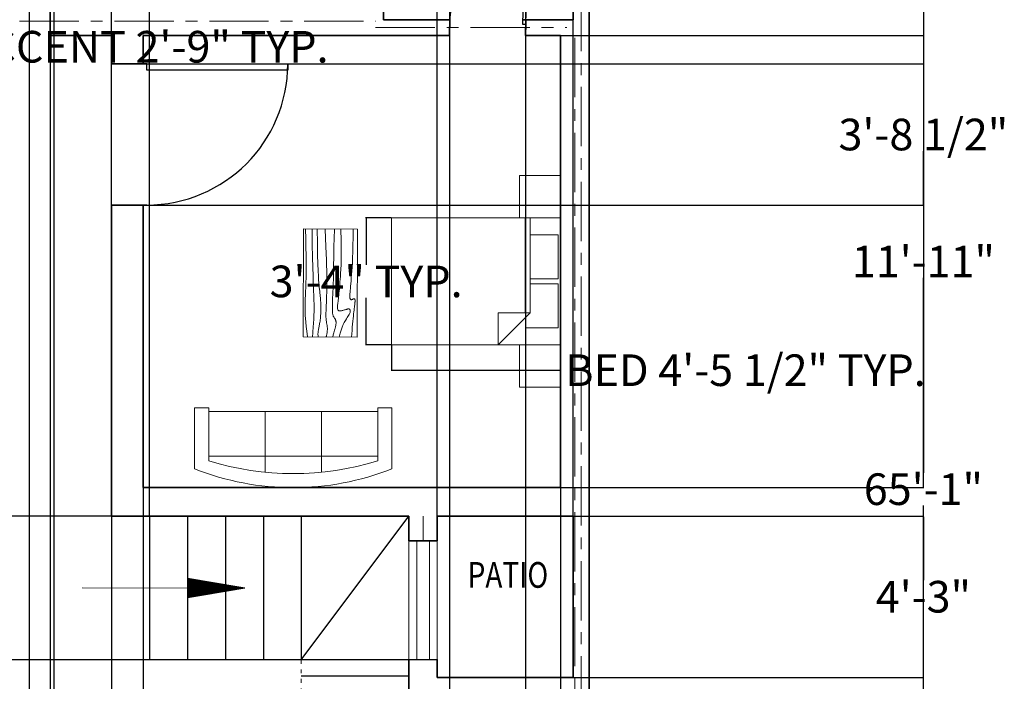
# Model space of a CAD drawing. Units: inches. Extents: x 541 to 1172, y -20 to 887.
# Tile 5 of 8: x 857 to 1169, y 378 to 588. Entities that reach past the tile are written whole.
import ezdxf

# ---------------------------------------------------------------- set-up
doc = ezdxf.new("R2010")
doc.units = ezdxf.units.IN
doc.header["$MEASUREMENT"] = 0
doc.linetypes.add('ACAD_ISO03W100', pattern=[30, 12, -18])
doc.linetypes.add('CENTER', pattern=[50.8, 31.75, -6.35, 6.35, -6.35])
doc.layers.get('0').update_dxf_attribs({"color": 70})
for name, color, linetype, lineweight in [('A-ANNO-DIMS', 2, 'Continuous', 18), ('A-ANNO-SYMB', 7, 'Continuous', 18), ('A-AREA-IDEN', 7, 'Continuous', 20), ('A-DOOR', 4, 'Continuous', 25), ('A-FLOR-STRS-HIDN', 131, 'ACAD_ISO03W100', 18), ('A-FURN', 30, 'Continuous', 18), ('A-WALL-CNTR', 1, 'CENTER', 13), ('STAIRS', 131, 'Continuous', 25), ('WALL', 7, 'Continuous', 35), ('WINDOW', 2, 'Continuous', 18)]:
    doc.layers.add(name, color=color, linetype=linetype, lineweight=lineweight)
doc.styles.get("Standard").update_dxf_attribs({"font": 'arial.ttf'})
doc.styles.add('YQ_DIM', font='SUPEROS.SHX', dxfattribs={"width": 0.8, "bigfont": 'HZDX.SHX'})
doc.dimstyles.get("Standard").update_dxf_attribs({"dimtxt": 10, "dimasz": 0.18, "dimexe": 0.18, "dimexo": 0.0625, "dimgap": 0.09, "dimtad": 0, "dimtih": 1, "dimtoh": 1, "dimdec": 1, "dimzin": 0, "dimdsep": 46, "dimlunit": 4, "dimtxsty": 'Standard', "dimcen": 0.09, "dimadec": 0, "dimazin": 0, "dimtfac": 1, "dimtdec": 1, "dimtofl": 0, "dimtmove": 0, "dimatfit": 3, "dimfxl": 1, "dimtolj": 1, "dimtzin": 0, "dimarcsym": 0})

# ---------------------------------------------------------------- blocks, each defined once
blk = doc.blocks.new('Bed - Queen')
for p, q in [((0, -80.00003), (0, 0)), ((0, 0), (59.99999, 0)), ((59.99999, 0), (59.99999, -80.00003)), ((7.99999, -1.2), (28.79998, -1.2)), ((7.99999, -14.4), (7.99999, -1.2)), ((28.79998, -1.2), (28.79998, -14.4)), ((31.19999, -1.2), (51.99999, -1.2)), ((31.19999, -14.4), (31.19999, -1.2)), ((51.99999, -1.2), (51.99999, -16.4)), ((0, -14.4), (44.8, -14.4)), ((44.8, -16.8), (0, -16.8)), ((59.99999, -29.6), (44.8, -14.4)), ((44.8, -14.4), (44.8, -29.6)), ((51.99999, -16.4), (46.79936, -16.4)), ((44.8, -29.6), (59.99999, -29.6)), ((59.99999, -80.00003), (0, -80.00003))]:
    blk.add_line(p, q)
blk = doc.blocks.new('Table - Rectangular Woodgrain 60 x 30 in.')
for p, q in [((0, 0), (0, -30)), ((60, 0), (0, 0)), ((60, -30), (60, 0)), ((0, -30), (60, -30))]:
    blk.add_line(p, q)
for points in [[(0, -2.4), (4.8155, -2.418), (9.0302, -2.4688), (12.709, -2.5477), (15.9167, -2.65), (18.7181, -2.7711), (21.1781, -2.9063), (23.3616, -3.0508), (25.3333, -3.2), (27.1477, -3.3495), (28.8172, -3.4958), (30.3437, -3.636), (31.7291, -3.7667), (32.9756, -3.8849), (34.0849, -3.9875), (35.059, -4.0714), (35.9, -4.1334), (36.6114, -4.1711), (37.2041, -4.1854), (37.6906, -4.1779), (38.0833, -4.15), (38.3948, -4.1034), (38.6375, -4.0396), (38.8239, -3.9602), (38.9666, -3.8667), (39.0764, -3.7608), (39.1573, -3.6448), (39.2116, -3.521), (39.2416, -3.3917), (39.2498, -3.2593), (39.2385, -3.1261), (39.21, -2.9944), (39.1666, -2.8667), (39.111, -2.7447), (39.0468, -2.6281), (38.978, -2.5163), (38.9083, -2.4083), (38.8418, -2.3035), (38.7823, -2.201), (38.7337, -2.1001), (38.7, -2), (38.6844, -1.9003), (38.6875, -1.8021), (38.7094, -1.707), (38.75, -1.6167), (38.8094, -1.5326), (38.8875, -1.4563), (38.9844, -1.3893), (39.1, -1.3333), (39.2351, -1.2896), (39.3937, -1.2583), (39.5804, -1.2396), (39.8, -1.2333), (40.057, -1.2396), (40.3562, -1.2583), (40.7023, -1.2896), (41.1, -1.3333), (41.5547, -1.3895), (42.0755, -1.4573), (42.6721, -1.5361), (43.3542, -1.625), (44.1316, -1.7233), (45.014, -1.8302), (46.0114, -1.9449), (47.1333, -2.0667), (48.3862, -2.1947), (49.7625, -2.3281), (51.2513, -2.4663), (52.8416, -2.6083), (54.5226, -2.7535), (56.2833, -2.9011), (58.1127, -3.0501), (60, -3.2)], [(0, -9.2), (6.5759, -9.0858), (11.9385, -9.0365), (16.2527, -9.0418), (19.6833, -9.0917), (22.3952, -9.1759), (24.5531, -9.2844), (26.322, -9.4069), (27.8666, -9.5333), (29.3241, -9.6553), (30.7203, -9.7719), (32.0532, -9.8837), (33.3208, -9.9917), (34.5213, -10.0965), (35.6526, -10.199), (36.7128, -10.2999), (37.7, -10.4), (38.6129, -10.4996), (39.4531, -10.5969), (40.223, -10.6895), (40.925, -10.775), (41.5613, -10.8512), (42.1344, -10.9156), (42.6465, -10.966), (43.1, -11), (43.4976, -11.0158), (43.8437, -11.0136), (44.143, -10.9942), (44.4, -10.9583), (44.6195, -10.9069), (44.8062, -10.8406), (44.9648, -10.7603), (45.1, -10.6667), (45.2155, -10.5598), (45.3114, -10.4365), (45.3871, -10.2929), (45.4416, -10.125), (45.4743, -9.929), (45.4844, -9.7011), (45.4709, -9.4371), (45.4333, -9.1333), (45.3716, -8.7883), (45.2896, -8.4104), (45.1919, -8.0107), (45.0833, -7.6), (44.9685, -7.1893), (44.8521, -6.7896), (44.7388, -6.4117), (44.6333, -6.0667), (44.54, -5.7628), (44.4614, -5.4979), (44.4001, -5.2675), (44.3583, -5.0667), (44.3384, -4.8909), (44.3427, -4.7354), (44.3736, -4.5956), (44.4333, -4.4667), (44.5236, -4.3453), (44.6427, -4.2333), (44.7884, -4.1339), (44.9583, -4.05), (45.1501, -3.9849), (45.3614, -3.9417), (45.59, -3.9234), (45.8333, -3.9333), (46.0915, -3.9749), (46.3734, -4.0531), (46.6906, -4.1736), (47.0542, -4.3417), (47.4756, -4.5629), (47.9661, -4.8427), (48.5372, -5.1866), (49.2, -5.6), (49.9676, -6.0844), (50.8594, -6.625), (51.8965, -7.2031), (53.1, -7.8), (54.491, -8.3969), (56.0906, -8.975), (57.9199, -9.5156), (60, -10)], [(0, -12.8), (5.1847, -12.9322), (9.6213, -13.0323), (13.3963, -13.1059), (16.5958, -13.1583), (19.3063, -13.1952), (21.614, -13.2219), (23.6054, -13.2439), (25.3666, -13.2667), (26.9728, -13.2947), (28.4531, -13.3281), (29.8256, -13.3663), (31.1083, -13.4083), (32.3191, -13.4535), (33.476, -13.501), (34.597, -13.5501), (35.7, -13.6), (36.7984, -13.6497), (37.8875, -13.6979), (38.9578, -13.743), (40, -13.7833), (41.0047, -13.8174), (41.9625, -13.8438), (42.864, -13.8607), (43.7, -13.8667), (44.4631, -13.8604), (45.1552, -13.8417), (45.7801, -13.8104), (46.3416, -13.7667), (46.8439, -13.7104), (47.2906, -13.6417), (47.6858, -13.5604), (48.0333, -13.4667), (48.3375, -13.3608), (48.6042, -13.2448), (48.8396, -13.121), (49.05, -12.9917), (49.2417, -12.8593), (49.4208, -12.7261), (49.5937, -12.5944), (49.7667, -12.4667), (49.9452, -12.3451), (50.1323, -12.2313), (50.3303, -12.1268), (50.5416, -12.0333), (50.7686, -11.9524), (51.0135, -11.8854), (51.2788, -11.8341), (51.5666, -11.8), (51.8785, -11.7843), (52.2116, -11.7865), (52.562, -11.8059), (52.926, -11.8417), (53.2998, -11.8931), (53.6795, -11.9594), (54.0614, -12.0397), (54.4416, -12.1333), (54.8223, -12.2401), (55.2293, -12.3625), (55.6942, -12.5037), (56.2489, -12.6667), (56.9251, -12.8547), (57.7545, -13.0708), (58.7689, -13.3182), (60, -13.6)], [(0, -18), (5.124, -17.7273), (9.6609, -17.5057), (13.6705, -17.3303), (17.2125, -17.1958), (20.3467, -17.0973), (23.1328, -17.0297), (25.6307, -16.9878), (27.9, -16.9667), (29.9928, -16.9617), (31.9302, -16.9703), (33.7254, -16.9907), (35.3917, -17.0208), (36.9423, -17.0588), (38.3906, -17.1026), (39.7499, -17.1503), (41.0333, -17.2), (42.2519, -17.2496), (43.4073, -17.2969), (44.4986, -17.3395), (45.525, -17.375), (46.4858, -17.4012), (47.3802, -17.4156), (48.2074, -17.416), (48.9667, -17.4), (49.6583, -17.3662), (50.2872, -17.3167), (50.8595, -17.2547), (51.3812, -17.1833), (51.8584, -17.1057), (52.2971, -17.025), (52.7034, -16.9443), (53.0833, -16.8667), (53.443, -16.7951), (53.789, -16.7313), (54.128, -16.6768), (54.4666, -16.6334), (54.8115, -16.6024), (55.1693, -16.5854), (55.5465, -16.5841), (55.95, -16.6), (56.3828, -16.6337), (56.8346, -16.6823), (57.2915, -16.7418), (57.7396, -16.8084), (58.165, -16.878), (58.5539, -16.9469), (58.8924, -17.0111), (59.1666, -17.0667), (59.3679, -17.1107), (59.5078, -17.1438), (59.6032, -17.1675), (59.6708, -17.1833), (59.7275, -17.193), (59.7901, -17.1979), (59.8753, -17.1998), (60, -17.2)], [(0, -22.4), (8.0098, -22.2501), (14.4094, -22.1011), (19.4168, -21.9535), (23.25, -21.8083), (26.1269, -21.6663), (28.2656, -21.5281), (29.884, -21.3947), (31.2, -21.2667), (32.3967, -21.1448), (33.5172, -21.0292), (34.5697, -20.9198), (35.5625, -20.8167), (36.5037, -20.7198), (37.4015, -20.6292), (38.2642, -20.5448), (39.1, -20.4667), (39.9164, -20.3951), (40.7187, -20.3313), (41.5117, -20.2768), (42.3, -20.2333), (43.0883, -20.2024), (43.8812, -20.1854), (44.6836, -20.1841), (45.5, -20.2), (46.3328, -20.234), (47.1747, -20.2844), (48.0163, -20.3488), (48.8479, -20.425), (49.66, -20.5106), (50.4429, -20.6031), (51.1872, -20.7004), (51.8833, -20.8), (52.5246, -20.8999), (53.1166, -20.9995), (53.6681, -21.0983), (54.1875, -21.1958), (54.6834, -21.2919), (55.1646, -21.3859), (55.6394, -21.4777), (56.1167, -21.5667), (56.6028, -21.6515), (57.0961, -21.7266), (57.5929, -21.7852), (58.0896, -21.8208), (58.5823, -21.8268), (59.0674, -21.7964), (59.5412, -21.723), (60, -21.6)], [(0, -25.2), (8.6355, -25.0504), (15.7026, -24.9031), (21.4049, -24.7606), (25.9458, -24.625), (29.529, -24.4988), (32.3578, -24.3844), (34.6359, -24.284), (36.5667, -24.2), (38.3213, -24.1341), (39.9417, -24.0854), (41.437, -24.0523), (42.8167, -24.0333), (44.0901, -24.0268), (45.2667, -24.0313), (46.3557, -24.0451), (47.3667, -24.0667), (48.309, -24.0947), (49.1928, -24.1287), (50.0284, -24.168), (50.826, -24.2125), (51.5959, -24.2617), (52.3483, -24.3151), (53.0935, -24.3725), (53.8417, -24.4334), (54.6009, -24.497), (55.3699, -24.561), (56.1454, -24.6226), (56.9239, -24.6792), (57.7021, -24.7279), (58.4764, -24.7662), (59.2435, -24.7911), (60, -24.8)], [(0, -28.8), (5.6867, -28.6681), (10.45, -28.5698), (14.407, -28.5012), (17.675, -28.4584), (20.3711, -28.4374), (22.6125, -28.4344), (24.5164, -28.4455), (26.2, -28.4667), (27.762, -28.4947), (29.2276, -28.5281), (30.6033, -28.5663), (31.8958, -28.6084), (33.1118, -28.6535), (34.2578, -28.7011), (35.3405, -28.7501), (36.3666, -28.8), (37.3443, -28.8497), (38.288, -28.8974), (39.2137, -28.9412), (40.1375, -28.9792), (41.0753, -29.0093), (42.0432, -29.0297), (43.0572, -29.0384), (44.1333, -29.0333), (45.2936, -29.0114), (46.5843, -28.9641), (48.0579, -28.8816), (49.7666, -28.7542), (51.7629, -28.5721), (54.0989, -28.3255), (56.8272, -28.0048), (60, -27.6)]]:
    blk.add_lwpolyline(points)
blk = doc.blocks.new('Sofa - Roundback 7 ft.')
for p, q in [((-12.00002, -32.4421), (-12.00003, -6.5971)), ((11.99997, -32.4421), (11.99998, -6.5971)), ((-36.000027, -34), (-36.000027, -11.4696)), ((35.99998, -34), (35.99998, -11.4696)), ((-35.999844, -13.3819), (35.9998, -13.3819)), ((-36.000027, -32.4421), (35.99998, -32.4421))]:
    blk.add_line(p, q)
for points in [[(-36.000027, -34), (-42.000027, -34), (-42.000027, -8)], [(41.99998, -8), (41.99998, -34), (35.99998, -34)]]:
    blk.add_lwpolyline(points)
for centre, radius, start, end in [((0, -114.25), 114.25, 68.43141, 111.5686), ((-0.00001, -127.1968), 121.1968, 72.72033, 107.2797)]:
    blk.add_arc(centre, radius, start, end)
blk = doc.blocks.new('*U25')
for p, q in [((-40, 0), (-40, 6)), ((0, 0), (0, 6))]:
    blk.add_line(p, q)
blk.add_lwpolyline([(0, 0), (0, -40), (-1.75, -40), (-1.75, 0)], close=True)
blk.add_arc((0, 0), 40, 180, 270)
blk = doc.blocks.new('*U23')
for p, q in [((0, 0), (0, -6)), ((40, 0), (40, -6))]:
    blk.add_line(p, q)
blk.add_lwpolyline([(0, 0), (0, 40), (1.75, 40), (1.75, 0)], close=True)
blk.add_arc((0, 0), 40, 0, 90)
blk = doc.blocks.new('FURN-NIGHTSTAND')
for p, q in [((0, 13.4), (0, 0)), ((0, 0), (13, 0))]:
    blk.add_line(p, q)
blk = doc.blocks.new('*D55')
at = {"layer": 'A-ANNO-DIMS', "color": 0, "lineweight": -2, "transparency": 16777216}
for p, q in [((974.8, 484.76), (974.8, 476.62)), ((1028.28, 484.76), (1028.28, 476.62)), ((974.98, 476.8), (1028.1, 476.8)), ((1028.28, 476.8), (1028.46, 476.8))]:
    blk.add_line(p, q, dxfattribs=at)
for points in [[(974.98, 476.83), (974.98, 476.77), (974.8, 476.8)], [(1028.1, 476.83), (1028.1, 476.77), (1028.28, 476.8)]]:
    blk.add_solid(points, dxfattribs=at)
at = {"layer": 'Defpoints', "color": 0, "lineweight": -2, "transparency": 16777216}
for p in [(974.8, 484.83), (1028.28, 484.83), (1028.28, 476.8)]:
    blk.add_point(p, dxfattribs=at)
at = {"layer": 'A-ANNO-DIMS', "color": 0, "transparency": 16777216, "insert": (1086.76, 476.8), "char_height": 10, "attachment_point": 5}
blk.add_mtext('\\A1;BED 4\'-5 1/2" TYP.', dxfattribs=at)
blk = doc.blocks.new('*D56')
at = {"layer": 'A-ANNO-DIMS', "color": 0, "lineweight": -2, "transparency": 16777216}
for p, q in [((974.74, 524.94), (966.6, 524.94)), ((966.78, 524.76), (966.78, 510.08)), ((966.78, 485.01), (966.78, 499.68)), ((974.74, 484.83), (966.6, 484.83))]:
    blk.add_line(p, q, dxfattribs=at)
for points in [[(966.75, 524.76), (966.81, 524.76), (966.78, 524.94)], [(966.75, 485.01), (966.81, 485.01), (966.78, 484.83)]]:
    blk.add_solid(points, dxfattribs=at)
at = {"layer": 'Defpoints', "color": 0, "lineweight": -2, "transparency": 16777216}
for p in [(974.8, 524.94), (966.78, 484.83), (974.8, 484.83)]:
    blk.add_point(p, dxfattribs=at)
at = {"layer": 'A-ANNO-DIMS', "color": 0, "transparency": 16777216, "insert": (966.78, 504.88), "char_height": 10, "attachment_point": 5}
blk.add_mtext('\\A1;3\'-4" TYP.', dxfattribs=at)
blk = doc.blocks.new('*D61')
at = {"layer": 'A-ANNO-DIMS', "color": 0, "lineweight": -2, "transparency": 16777216}
for p, q in [((802.49, 574.25), (802.49, 579.28)), ((835.27, 574.25), (835.27, 579.28)), ((802.67, 579.1), (835.09, 579.1)), ((835.27, 579.1), (835.45, 579.1))]:
    blk.add_line(p, q, dxfattribs=at)
for points in [[(802.67, 579.13), (802.67, 579.07), (802.49, 579.1)], [(835.09, 579.13), (835.09, 579.07), (835.27, 579.1)]]:
    blk.add_solid(points, dxfattribs=at)
at = {"layer": 'Defpoints', "color": 0, "lineweight": -2, "transparency": 16777216}
for p in [(835.27, 579.1), (802.49, 574.19), (835.27, 574.19)]:
    blk.add_point(p, dxfattribs=at)
at = {"layer": 'A-ANNO-DIMS', "color": 0, "transparency": 16777216, "insert": (896.96, 579.1), "char_height": 10, "attachment_point": 5}
blk.add_mtext('\\A1;ACCENT 2\'-9" TYP.', dxfattribs=at)
blk = doc.blocks.new('*D70')
at = {"layer": 'A-ANNO-DIMS', "color": 0, "lineweight": -2, "transparency": 16777216}
for p, q in [((1036.7, 829.68), (1143.21, 829.68)), ((1143.03, 829.5), (1143.03, 444.36)), ((1143.03, 48.83), (1143.03, 433.97)), ((1037.35, 48.65), (1143.21, 48.65))]:
    blk.add_line(p, q, dxfattribs=at)
for points in [[(1143, 829.5), (1143.06, 829.5), (1143.03, 829.68)], [(1143, 48.83), (1143.06, 48.83), (1143.03, 48.65)]]:
    blk.add_solid(points, dxfattribs=at)
at = {"layer": 'Defpoints', "color": 0, "lineweight": -2, "transparency": 16777216}
for p in [(1036.64, 829.68), (1037.28, 48.65), (1143.03, 48.65)]:
    blk.add_point(p, dxfattribs=at)
at = {"layer": 'A-ANNO-DIMS', "color": 0, "transparency": 16777216, "insert": (1143.03, 439.17), "char_height": 10, "attachment_point": 5}
blk.add_mtext('\\A1;65\'-1"', dxfattribs=at)
blk = doc.blocks.new('*D86')
at = {"layer": 'A-ANNO-DIMS', "color": 0, "lineweight": -2, "transparency": 16777216}
for p, q in [((896.28, 439.59), (896.28, -5.37)), ((1028.28, 439.59), (1028.28, -5.37)), ((896.46, -5.19), (945.49, -5.19)), ((1028.1, -5.19), (979.08, -5.19))]:
    blk.add_line(p, q, dxfattribs=at)
for points in [[(896.46, -5.16), (896.46, -5.22), (896.28, -5.19)], [(1028.1, -5.16), (1028.1, -5.22), (1028.28, -5.19)]]:
    blk.add_solid(points, dxfattribs=at)
at = {"layer": 'Defpoints', "color": 0, "lineweight": -2, "transparency": 16777216}
for p in [(896.28, 439.65), (1028.28, 439.65), (1028.28, -5.19)]:
    blk.add_point(p, dxfattribs=at)
at = {"layer": 'A-ANNO-DIMS', "color": 0, "transparency": 16777216, "insert": (962.28, -5.19), "char_height": 10, "attachment_point": 5}
blk.add_mtext('\\A1;11\'-0"', dxfattribs=at)
blk = doc.blocks.new('*D87')
at = {"layer": 'A-ANNO-DIMS', "color": 0, "lineweight": -2, "transparency": 16777216}
for p, q in [((1028.35, 582.65), (1143.21, 582.65)), ((1143.03, 582.47), (1143.03, 516.26)), ((1143.03, 439.83), (1143.03, 506.04)), ((1028.35, 439.65), (1143.21, 439.65))]:
    blk.add_line(p, q, dxfattribs=at)
for points in [[(1143, 582.47), (1143.06, 582.47), (1143.03, 582.65)], [(1143, 439.83), (1143.06, 439.83), (1143.03, 439.65)]]:
    blk.add_solid(points, dxfattribs=at)
at = {"layer": 'Defpoints', "color": 0, "lineweight": -2, "transparency": 16777216}
for p in [(1028.28, 582.65), (1143.03, 582.65), (1028.28, 439.65)]:
    blk.add_point(p, dxfattribs=at)
at = {"layer": 'A-ANNO-DIMS', "color": 0, "transparency": 16777216, "insert": (1143.03, 511.15), "char_height": 10, "attachment_point": 5}
blk.add_mtext('\\A1;11\'-11"', dxfattribs=at)
blk = doc.blocks.new('*D88')
at = {"layer": 'A-ANNO-DIMS', "color": 0, "lineweight": -2, "transparency": 16777216}
for p, q in [((1032.35, 430.65), (1143.21, 430.65)), ((1143.03, 430.47), (1143.03, 410.35)), ((1143.03, 379.83), (1143.03, 399.96)), ((1032.35, 379.65), (1143.21, 379.65))]:
    blk.add_line(p, q, dxfattribs=at)
for points in [[(1143, 430.47), (1143.06, 430.47), (1143.03, 430.65)], [(1143, 379.83), (1143.06, 379.83), (1143.03, 379.65)]]:
    blk.add_solid(points, dxfattribs=at)
at = {"layer": 'Defpoints', "color": 0, "lineweight": -2, "transparency": 16777216}
for p in [(1032.28, 430.65), (1032.28, 379.65), (1143.03, 379.65)]:
    blk.add_point(p, dxfattribs=at)
at = {"layer": 'A-ANNO-DIMS', "color": 0, "transparency": 16777216, "insert": (1143.03, 405.15), "char_height": 10, "attachment_point": 5}
blk.add_mtext('\\A1;4\'-3"', dxfattribs=at)
blk = doc.blocks.new('*D89')
at = {"layer": 'A-ANNO-DIMS', "color": 0, "lineweight": -2, "transparency": 16777216}
for p, q in [((989.28, 430.72), (989.28, 872.66)), ((989.46, 872.48), (997.41, 872.48)), ((1032.1, 872.48), (1024.16, 872.48)), ((1032.28, 430.72), (1032.28, 872.66))]:
    blk.add_line(p, q, dxfattribs=at)
for points in [[(989.46, 872.51), (989.46, 872.45), (989.28, 872.48)], [(1032.1, 872.51), (1032.1, 872.45), (1032.28, 872.48)]]:
    blk.add_solid(points, dxfattribs=at)
at = {"layer": 'Defpoints', "color": 0, "lineweight": -2, "transparency": 16777216}
for p in [(1032.28, 872.48), (989.28, 430.65), (1032.28, 430.65)]:
    blk.add_point(p, dxfattribs=at)
at = {"layer": 'A-ANNO-DIMS', "color": 0, "transparency": 16777216, "insert": (1010.78, 872.48), "char_height": 10, "attachment_point": 5}
blk.add_mtext('\\A1;3\'-7"', dxfattribs=at)
blk = doc.blocks.new('*D95')
at = {"layer": 'A-ANNO-DIMS', "color": 0, "lineweight": -2, "transparency": 16777216}
for p, q in [((886.28, 385.11), (886.28, -5.37)), ((980.28, 385.11), (980.28, -5.37)), ((886.46, -5.19), (916.06, -5.19)), ((980.1, -5.19), (950.51, -5.19))]:
    blk.add_line(p, q, dxfattribs=at)
for points in [[(886.46, -5.16), (886.46, -5.22), (886.28, -5.19)], [(980.1, -5.16), (980.1, -5.22), (980.28, -5.19)]]:
    blk.add_solid(points, dxfattribs=at)
at = {"layer": 'Defpoints', "color": 0, "lineweight": -2, "transparency": 16777216}
for p in [(886.28, 385.17), (980.28, 385.17), (980.28, -5.19)]:
    blk.add_point(p, dxfattribs=at)
at = {"layer": 'A-ANNO-DIMS', "color": 0, "transparency": 16777216, "insert": (933.28, -5.19), "char_height": 10, "attachment_point": 5}
blk.add_mtext('\\A1;7\'-10"', dxfattribs=at)
blk = doc.blocks.new('*D96')
at = {"layer": 'A-ANNO-DIMS', "color": 0, "lineweight": -2, "transparency": 16777216}
for p, q in [((980.22, 430.65), (573.66, 430.65)), ((573.84, 430.47), (573.84, 413.18)), ((573.84, 385.35), (573.84, 402.65)), ((980.22, 385.17), (573.66, 385.17))]:
    blk.add_line(p, q, dxfattribs=at)
for points in [[(573.81, 430.47), (573.87, 430.47), (573.84, 430.65)], [(573.81, 385.35), (573.87, 385.35), (573.84, 385.17)]]:
    blk.add_solid(points, dxfattribs=at)
at = {"layer": 'Defpoints', "color": 0, "lineweight": -2, "transparency": 16777216}
for p in [(573.84, 430.65), (980.28, 430.65), (980.28, 385.17)]:
    blk.add_point(p, dxfattribs=at)
at = {"layer": 'A-ANNO-DIMS', "color": 0, "transparency": 16777216, "insert": (573.84, 407.91), "char_height": 10, "attachment_point": 5}
blk.add_mtext('\\A1;3\'-9 1/2"', dxfattribs=at)
blk = doc.blocks.new('*D97')
at = {"layer": 'A-ANNO-DIMS', "color": 0, "lineweight": -2, "transparency": 16777216}
for p, q in [((886.28, 430.72), (886.28, 872.66)), ((886.46, 872.48), (898.1, 872.48)), ((898.28, 430.72), (898.28, 872.66)), ((898.28, 872.48), (898.46, 872.48))]:
    blk.add_line(p, q, dxfattribs=at)
for points in [[(886.46, 872.51), (886.46, 872.45), (886.28, 872.48)], [(898.1, 872.51), (898.1, 872.45), (898.28, 872.48)]]:
    blk.add_solid(points, dxfattribs=at)
at = {"layer": 'Defpoints', "color": 0, "lineweight": -2, "transparency": 16777216}
for p in [(898.28, 872.48), (886.28, 430.65), (898.28, 430.65)]:
    blk.add_point(p, dxfattribs=at)
at = {"layer": 'A-ANNO-DIMS', "color": 0, "transparency": 16777216, "insert": (911.37, 872.48), "char_height": 10, "attachment_point": 5}
blk.add_mtext('\\A1;1\'-0"', dxfattribs=at)
blk = doc.blocks.new('*D98')
at = {"layer": 'A-ANNO-DIMS', "color": 0, "lineweight": -2, "transparency": 16777216}
for p, q in [((993.28, 326.72), (993.28, 872.66)), ((993.46, 872.48), (1017.14, 872.48)), ((1017.32, 326.72), (1017.32, 872.66)), ((1017.32, 872.48), (1017.5, 872.48))]:
    blk.add_line(p, q, dxfattribs=at)
for points in [[(993.46, 872.51), (993.46, 872.45), (993.28, 872.48)], [(1017.14, 872.51), (1017.14, 872.45), (1017.32, 872.48)]]:
    blk.add_solid(points, dxfattribs=at)
at = {"layer": 'Defpoints', "color": 0, "lineweight": -2, "transparency": 16777216}
for p in [(1017.32, 872.48), (993.28, 326.65), (1017.32, 326.65)]:
    blk.add_point(p, dxfattribs=at)
at = {"layer": 'A-ANNO-DIMS', "color": 0, "transparency": 16777216, "insert": (1030.97, 872.48), "char_height": 10, "attachment_point": 5}
blk.add_mtext('\\A1;2\'-0"', dxfattribs=at)
blk = doc.blocks.new('*D102')
at = {"layer": 'A-ANNO-DIMS', "color": 0, "lineweight": -2, "transparency": 16777216}
for p, q in [((822.26, 582.59), (822.26, -5.37)), ((866.83, 582.59), (866.83, -5.37)), ((822.44, -5.19), (866.65, -5.19)), ((866.83, -5.19), (867.01, -5.19))]:
    blk.add_line(p, q, dxfattribs=at)
for points in [[(822.44, -5.16), (822.44, -5.22), (822.26, -5.19)], [(866.65, -5.16), (866.65, -5.22), (866.83, -5.19)]]:
    blk.add_solid(points, dxfattribs=at)
at = {"layer": 'Defpoints', "color": 0, "lineweight": -2, "transparency": 16777216}
for p in [(822.26, 582.65), (866.83, 582.65), (866.83, -5.19)]:
    blk.add_point(p, dxfattribs=at)
at = {"layer": 'A-ANNO-DIMS', "color": 0, "transparency": 16777216, "insert": (892.04, -5.19), "char_height": 10, "attachment_point": 5}
blk.add_mtext('\\A1;3\'-8 1/2"', dxfattribs=at)
blk = doc.blocks.new('*D103')
at = {"layer": 'A-ANNO-DIMS', "color": 0, "lineweight": -2, "transparency": 16777216}
for p, q in [((896.35, 573.65), (1143.21, 573.65)), ((1143.03, 573.47), (1143.03, 556.61)), ((1143.03, 529.22), (1143.03, 546.08)), ((896.35, 529.04), (1143.21, 529.04))]:
    blk.add_line(p, q, dxfattribs=at)
for points in [[(1143, 573.47), (1143.06, 573.47), (1143.03, 573.65)], [(1143, 529.22), (1143.06, 529.22), (1143.03, 529.04)]]:
    blk.add_solid(points, dxfattribs=at)
at = {"layer": 'Defpoints', "color": 0, "lineweight": -2, "transparency": 16777216}
for p in [(896.28, 573.65), (896.28, 529.04), (1143.03, 529.04)]:
    blk.add_point(p, dxfattribs=at)
at = {"layer": 'A-ANNO-DIMS', "color": 0, "transparency": 16777216, "insert": (1143.03, 551.34), "char_height": 10, "attachment_point": 5}
blk.add_mtext('\\A1;3\'-8 1/2"', dxfattribs=at)
blk = doc.blocks.new('*D104')
at = {"layer": 'A-ANNO-DIMS', "color": 0, "lineweight": -2, "transparency": 16777216}
for p, q in [((860.28, 177.72), (860.28, 872.66)), ((860.46, 872.48), (867.98, 872.48)), ((868.16, 177.72), (868.16, 872.66)), ((868.16, 872.48), (868.34, 872.48))]:
    blk.add_line(p, q, dxfattribs=at)
for points in [[(860.46, 872.51), (860.46, 872.45), (860.28, 872.48)], [(867.98, 872.51), (867.98, 872.45), (868.16, 872.48)]]:
    blk.add_solid(points, dxfattribs=at)
at = {"layer": 'Defpoints', "color": 0, "lineweight": -2, "transparency": 16777216}
for p in [(868.16, 872.48), (860.28, 177.65), (868.16, 177.65)]:
    blk.add_point(p, dxfattribs=at)
at = {"layer": 'A-ANNO-DIMS', "color": 0, "transparency": 16777216, "insert": (881.72, 872.48), "char_height": 10, "attachment_point": 5}
blk.add_mtext('\\A1;0\'-8"', dxfattribs=at)

msp = doc.modelspace()

# ---------------------------------------------------------------- linework, layer by layer
at = {"layer": 'A-ANNO-SYMB'}
msp.add_line((876.98, 408.01), (910.28, 407.91), dxfattribs=at)
msp.add_lwpolyline([(910.28, 407.91, 6.46, 0.327, 0), (928.42, 407.91, 0, 0, 0)], format="xyseb", dxfattribs=at)
at = {"layer": 'A-FLOR-STRS-HIDN', "ltscale": 0.1}
msp.add_lwpolyline([(946.28, 385.17), (946.28, 375.17), (980.28, 330.65)], dxfattribs=at)
at = {"layer": 'A-WALL-CNTR', "ltscale": 0.590551}
for p, q in [((1034.78, 247.65), (1034.78, 712.65)), ((797.19, 587.15), (969.78, 587.15)), ((969.78, 585.15), (1030.28, 585.15)), ((1032.78, 173.15), (1032.78, 585.15)), ((984.78, 422.78), (984.78, 430.65))]:
    msp.add_line(p, q, dxfattribs=at)
at = {"layer": 'STAIRS'}
for p, q in [((886.28, 430.65), (886.28, 385.17)), ((898.28, 430.65), (898.28, 385.17)), ((910.28, 430.65), (910.28, 385.17)), ((922.28, 430.65), (922.28, 385.17)), ((934.28, 430.65), (934.28, 385.17)), ((946.28, 430.65), (946.28, 385.17)), ((946.28, 385.17), (980.28, 430.65)), ((980.28, 385.17), (886.28, 385.17)), ((946.28, 380.17), (980.28, 380.17))]:
    msp.add_line(p, q, dxfattribs=at)
at = {"layer": 'WALL'}
for p, q in [((1037.28, 48.65), (1037.28, 712.65)), ((972.28, 587.65), (972.28, 647.65)), ((1032.28, 587.65), (1032.28, 647.65)), ((866.83, 591.65), (866.83, 582.65)), ((972.28, 587.65), (993.27, 587.65)), ((993.27, 587.65), (993.15, 583.3)), ((1016.27, 587.65), (1032.28, 587.65)), ((1017.32, 587.65), (1017.18, 582.65)), ((866.83, 582.65), (886.28, 582.65)), ((886.28, 573.65), (886.28, 582.65)), ((896.28, 582.65), (993.15, 582.65)), ((993.15, 583.3), (993.15, 582.65)), ((1017.18, 582.65), (1028.28, 582.65)), ((1028.28, 439.65), (1028.28, 582.65)), ((896.28, 573.65), (886.28, 573.65)), ((886.28, 473.81), (886.28, 529.04)), ((896.28, 529.04), (886.28, 529.04)), ((980.28, 422.78), (980.28, 430.65)), ((989.28, 422.78), (989.28, 430.65)), ((989.28, 430.65), (1032.28, 430.65)), ((1032.28, 379.65), (1032.28, 430.65)), ((989.28, 422.78), (980.28, 422.78)), ((980.28, 385.17), (989.28, 385.34)), ((980.28, 363.73), (980.28, 385.17)), ((989.28, 385.34), (989.28, 379.65)), ((989.28, 379.65), (1032.28, 379.65))]:
    msp.add_line(p, q, dxfattribs=at)
for points in [[(896.28, 573.65), (896.28, 582.65)], [(1028.28, 439.65), (896.28, 439.65), (896.28, 529.04)], [(886.28, 475.81), (886.28, 430.65), (887.28, 430.65), (980.28, 430.65)]]:
    msp.add_lwpolyline(points, dxfattribs=at)
at = {"layer": 'WINDOW'}
for p, q in [((980.28, 422.78), (980.28, 385.17)), ((982.78, 422.78), (982.78, 385.25)), ((986.78, 422.78), (986.78, 385.25)), ((989.28, 422.78), (989.28, 385.34))]:
    msp.add_line(p, q, dxfattribs=at)

# ---------------------------------------------------------------- block references
at = {"layer": 'A-DOOR'}
for name, p, xscale, yscale, zscale, rotation in [('*U23', (1017.28, 586.26), -0.6011813567709343, 0.6011813567709343, 0.6011813567709343, 358.4510988302025), ('*U25', (897.38, 573.65), 1.115231810502029, 1.115231810502029, 1.115231810502029, 90)]:
    msp.add_blockref(name, p, dxfattribs=dict(at, xscale=xscale, yscale=yscale, zscale=zscale, rotation=rotation))
at = {"layer": 'A-FURN', "extrusion": (0, 0, -1), "zscale": -1, "rotation": 180}
msp.add_blockref('FURN-NIGHTSTAND', (-1015.28, 538.33), dxfattribs=at)
at = {"layer": 'A-FURN'}
for name, p, xscale, yscale, zscale, rotation in [('Bed - Queen', (1028.28, 524.94), 0.6685054037368693, 0.6685054037368693, 0.6685054037368693, 270), ('Table - Rectangular Woodgrain 60 x 30 in.', (964.03, 521.44), 0.5694163205475999, 0.5694163205475999, 0.5694163205475999, 269.908106286482), ('Sofa - Roundback 7 ft.', (943.71, 439.65), 0.7424226432878923, 0.7424226432878923, 0.7424226432878923, 180)]:
    msp.add_blockref(name, p, dxfattribs=dict(at, xscale=xscale, yscale=yscale, zscale=zscale, rotation=rotation))
msp.add_blockref('FURN-NIGHTSTAND', (1015.28, 471.43), dxfattribs=at)

# ---------------------------------------------------------------- texts
at = {"layer": 'A-AREA-IDEN', "style": 'YQ_DIM', "width": 0.8}
msp.add_text(' PATIO', height=8.13, dxfattribs=at).set_placement((996.88, 407.99))

# ---------------------------------------------------------------- dimensions: what is measured, and where the dimension line sits
at = {"layer": 'A-ANNO-DIMS'}
for base, p1, p2, picture, middle in [((868.16, 872.48), (860.28, 177.65), (868.16, 177.65), '*D104', (881.72, 872.48)), ((898.28, 872.48), (886.28, 430.65), (898.28, 430.65), '*D97', (911.37, 872.48)), ((1032.28, 872.48), (989.28, 430.65), (1032.28, 430.65), '*D89', (1010.78, 872.48)), ((1017.32, 872.48), (993.27, 326.65), (1017.32, 326.65), '*D98', (1030.97, 872.48)), ((866.83, -5.19), (822.26, 582.65), (866.83, 582.65), '*D102', (892.04, -5.19)), ((1028.28, -5.19), (896.28, 439.65), (1028.28, 439.65), '*D86', (962.28, -5.19)), ((980.28, -5.19), (886.28, 385.17), (980.28, 385.17), '*D95', (933.28, -5.19))]:
    dim = msp.add_linear_dim(base=base, p1=p1, p2=p2, dimstyle='Standard', override={"dimdec": 1, "dimlfac": 1, "dimrnd": 0, "dimzin": 1, "dimdsep": 46, "dimlunit": 4, "dimfrac": 2}, dxfattribs=at)
    dim.commit()
    dim.dimension.update_dxf_attribs({"geometry": picture, "text_midpoint": middle})
for base, p1, p2, picture, middle in [((1143.03, 48.65), (1036.64, 829.68), (1037.28, 48.65), '*D70', (1143.03, 439.17)), ((1143.03, 582.65), (1028.28, 439.65), (1028.28, 582.65), '*D87', (1143.03, 511.15)), ((1143.03, 529.04), (896.28, 573.65), (896.28, 529.04), '*D103', (1143.03, 551.34)), ((573.84, 430.65), (980.28, 385.17), (980.28, 430.65), '*D96', (573.84, 407.91)), ((1143.03, 379.65), (1032.28, 430.65), (1032.28, 379.65), '*D88', (1143.03, 405.15))]:
    dim = msp.add_linear_dim(base=base, p1=p1, p2=p2, angle=90, dimstyle='Standard', override={"dimdec": 1, "dimlfac": 1, "dimrnd": 0, "dimzin": 1, "dimdsep": 46, "dimlunit": 4, "dimfrac": 2}, dxfattribs=at)
    dim.commit()
    dim.dimension.update_dxf_attribs({"geometry": picture, "text_midpoint": middle})
for base, p1, p2, text, picture, middle in [((835.27, 579.1), (802.49, 574.19), (835.27, 574.19), 'ACCENT <> TYP.', '*D61', (896.96, 579.1)), ((1028.28, 476.8), (974.8, 484.83), (1028.28, 484.83), 'BED <> TYP.', '*D55', (1086.76, 476.8))]:
    dim = msp.add_linear_dim(base=base, p1=p1, p2=p2, text=text, dimstyle='Standard', override={"dimdec": 1, "dimlfac": 1, "dimrnd": 0, "dimzin": 1, "dimdsep": 46, "dimlunit": 4, "dimfrac": 2}, dxfattribs=at)
    dim.commit()
    dim.dimension.update_dxf_attribs({"geometry": picture, "text_midpoint": middle})
dim = msp.add_linear_dim(base=(966.78, 484.83), p1=(974.8, 524.94), p2=(974.8, 484.83), angle=270, text='<> TYP.', dimstyle='Standard', override={"dimdec": 1, "dimlfac": 1, "dimrnd": 0, "dimzin": 1, "dimdsep": 46, "dimlunit": 4, "dimfrac": 2}, dxfattribs=at)
dim.commit()
dim.dimension.update_dxf_attribs({"geometry": '*D56', "text_midpoint": (966.78, 504.88)})

doc.saveas('drawing.dxf')
